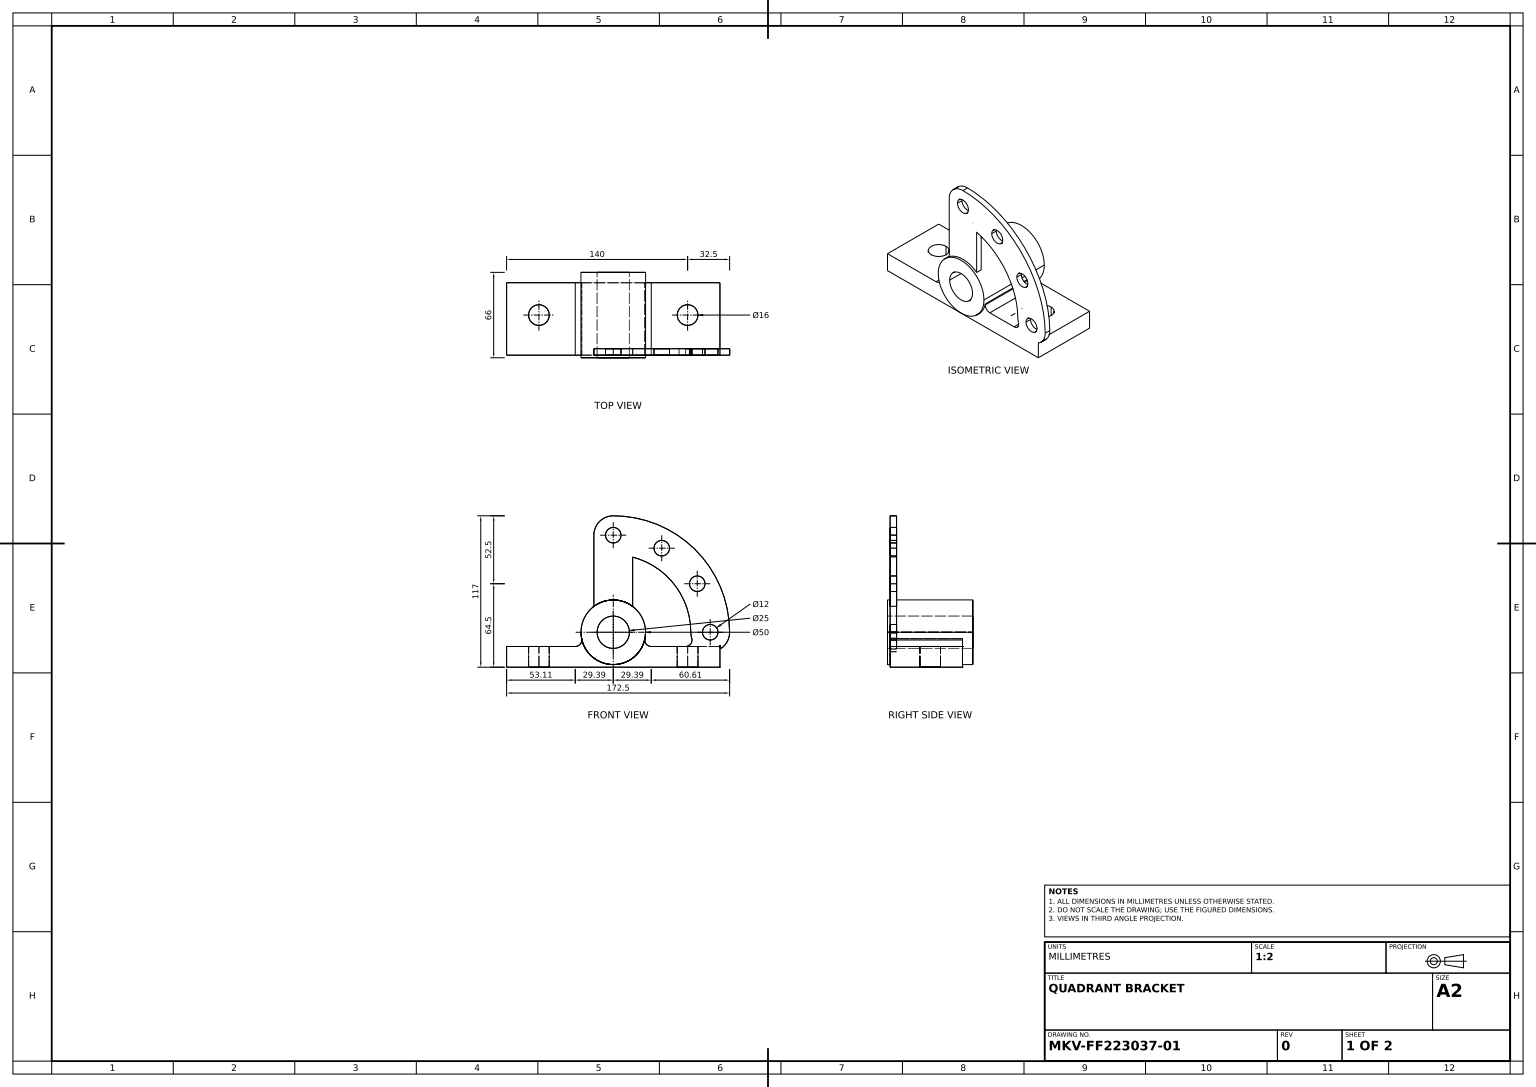
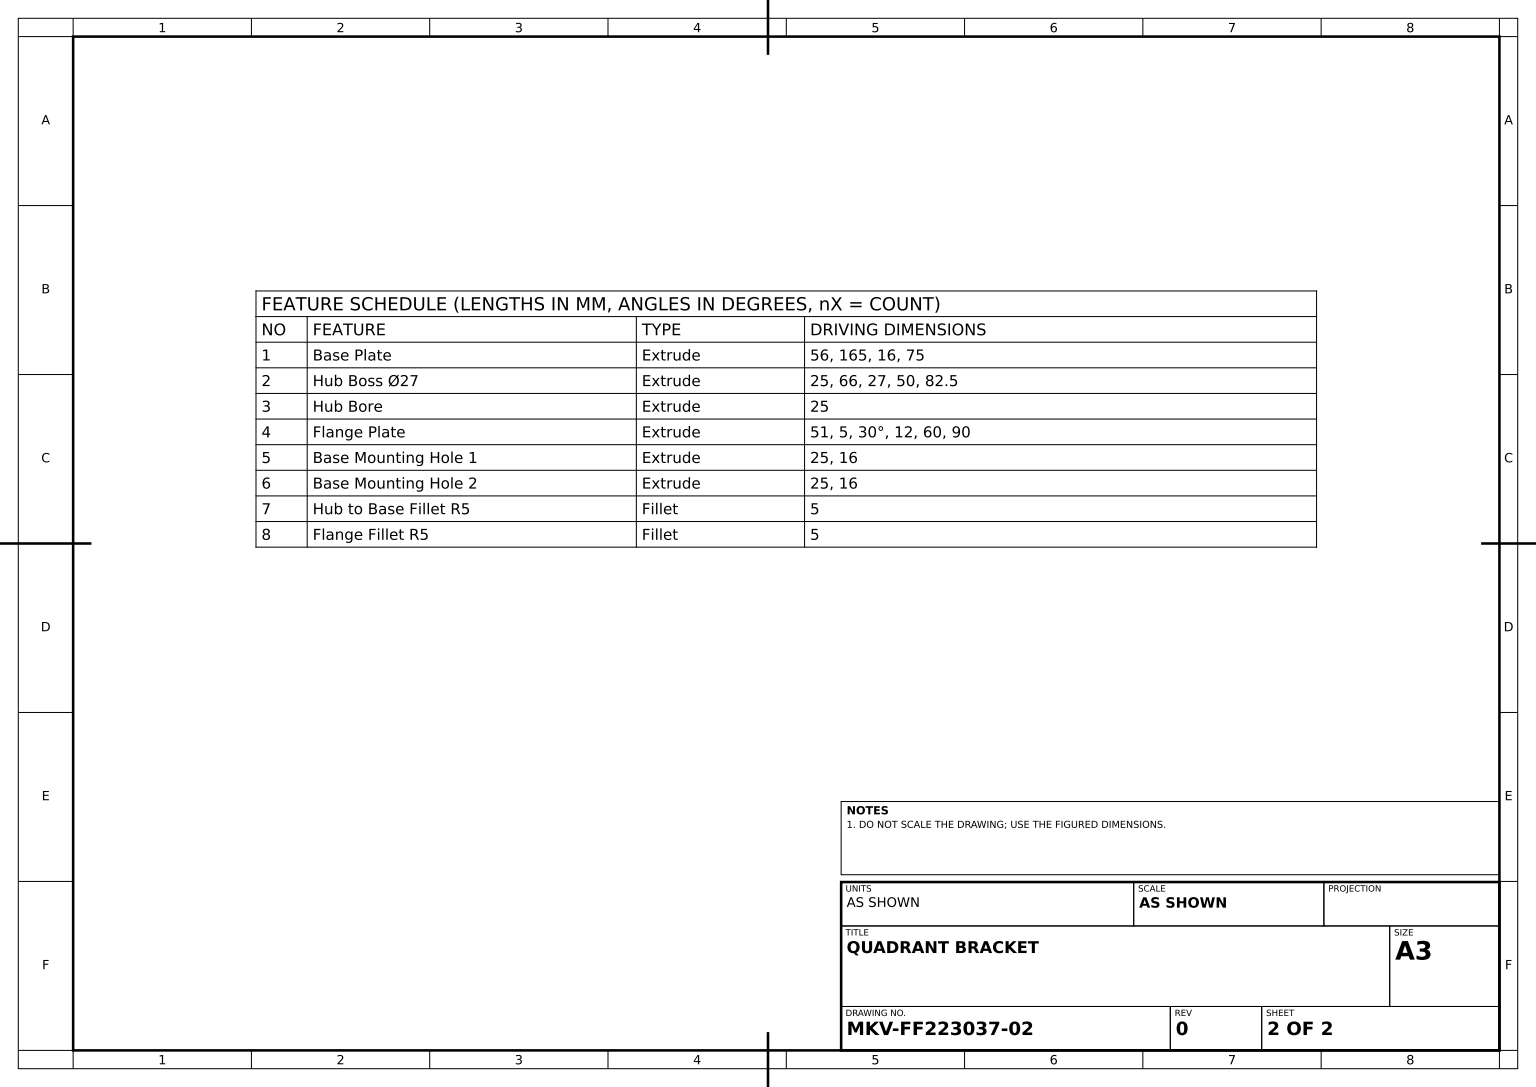
from build123d import *

# Parameters (mm, degrees)
BASE_PLATE_DEPTH               = 56
HUB_BOSS_PROFILE_R             = 25
HUB_BOSS_PROFILE_R_2           = 12.5
HUB_BOSS_27_DEPTH              = 33
HUB_BORE_PROFILE_R             = 12.5
HUB_BORE_DEPTH                 = 186.162091153
FLANGE_START                   = 5
FLANGE_PLATE_PROFILE_R         = 6
FLANGE_PLATE_DEPTH             = 5
BASE_MOUNTING_HOLE_1_PROFILE_R = 8
BASE_MOUNTING_HOLE_1_DEPTH     = 209.137574695
BASE_MOUNTING_HOLE_2_PROFILE_R = 8
BASE_MOUNTING_HOLE_2_DEPTH     = 209.137574695
HUB_TO_BASE_FILLET_R5_R        = 5
FLANGE_FILLET_R5_R             = 5


with BuildPart() as part:
    # Base Plate Profile → Base Plate (new body)
    with BuildSketch(Plane.XY):
        Polygon((0, 0), (75, 0), (165, 0), (165, 16), (0, 16), align=None)
    extrude(amount=BASE_PLATE_DEPTH)

    # Hub Boss Profile → Hub Boss Ø27 (add, symmetric)
    with BuildSketch(Plane.XY.offset(25)):
        with Locations((82.5, 27)):
            Circle(HUB_BOSS_PROFILE_R)
        with Locations((82.5, 27)):
            Circle(HUB_BOSS_PROFILE_R_2, mode=Mode.SUBTRACT)
    extrude(amount=HUB_BOSS_27_DEPTH, both=True)

    # Hub Bore Profile → Hub Bore (cut, through all)
    with BuildSketch(Plane.XY.offset(58)):
        with Locations((82.5, 27)):
            Circle(HUB_BORE_PROFILE_R)
    extrude(amount=-HUB_BORE_DEPTH, mode=Mode.SUBTRACT)

    # Flange Plate Profile → Flange Plate (add)
    # profile 1 of 2: a face of its own
    with BuildSketch(Plane.XY.offset(51).offset(FLANGE_START)):
        with BuildLine():
            ThreePointArc((82.5, 87), (71.893398282, 91.393398282), (67.5, 102))
            Line((67.5, 102), (67.5, 47))
            ThreePointArc((67.5, 47), (82.5, 52), (97.5, 47))
            Line((97.5, 47), (97.5, 85.094750193))
            ThreePointArc((97.5, 85.094750193), (90.060257549, 86.521781776), (82.5, 87))
        make_face()
    # profile 2 of 2: a face of its own
    with BuildSketch(Plane.XY.offset(51).offset(FLANGE_START)):
        with BuildLine():
            ThreePointArc((142.5, 27), (124.926406871, 69.426406871), (82.5, 87))
            ThreePointArc((82.5, 87), (67.5, 102), (82.5, 117))
            ThreePointArc((82.5, 117), (146.139610307, 90.639610307), (172.5, 27))
            ThreePointArc((172.5, 27), (157.5, 12), (142.5, 27))
        make_face()
        with Locations((120, 91.951905284)):
            Circle(FLANGE_PLATE_PROFILE_R, mode=Mode.SUBTRACT)
        with Locations((147.451905284, 64.5)):
            Circle(FLANGE_PLATE_PROFILE_R, mode=Mode.SUBTRACT)
        with Locations((157.5, 27)):
            Circle(FLANGE_PLATE_PROFILE_R, mode=Mode.SUBTRACT)
        with Locations((82.5, 102)):
            Circle(FLANGE_PLATE_PROFILE_R, mode=Mode.SUBTRACT)
    extrude(amount=-FLANGE_PLATE_DEPTH)

    # Base Mounting Hole 1 Profile → Base Mounting Hole 1 (cut, through all)
    with BuildSketch(Plane(origin=(0, 16, 0), x_dir=(1, 0, 0), z_dir=(0, 1, 0))):
        with Locations(Location((25, -25, 0), (0, 0, 270))):
            Circle(BASE_MOUNTING_HOLE_1_PROFILE_R)
    extrude(amount=-BASE_MOUNTING_HOLE_1_DEPTH, mode=Mode.SUBTRACT)

    # Base Mounting Hole 2 Profile → Base Mounting Hole 2 (cut, through all)
    with BuildSketch(Plane(origin=(0, 16, 0), x_dir=(1, 0, 0), z_dir=(0, 1, 0))):
        with Locations(Location((140, -25, 0), (0, 0, 270))):
            Circle(BASE_MOUNTING_HOLE_2_PROFILE_R)
    extrude(amount=-BASE_MOUNTING_HOLE_2_DEPTH, mode=Mode.SUBTRACT)

    # Hub to Base Fillet R5
    hub_to_base_fillet_r5_edges = [part.edges().sort_by_distance(p)[0] for p in [
        (60.050055679, 16, 28),
    ]]
    fillet(hub_to_base_fillet_r5_edges, radius=HUB_TO_BASE_FILLET_R5_R)

    # Flange Fillet R5
    flange_fillet_r5_edges = [part.edges().sort_by_distance(p)[0] for p in [
        (104.949944321, 16, 28),
        (147.301960973, 16, 53.5),
    ]]
    fillet(flange_fillet_r5_edges, radius=FLANGE_FILLET_R5_R)


solid = part.part
